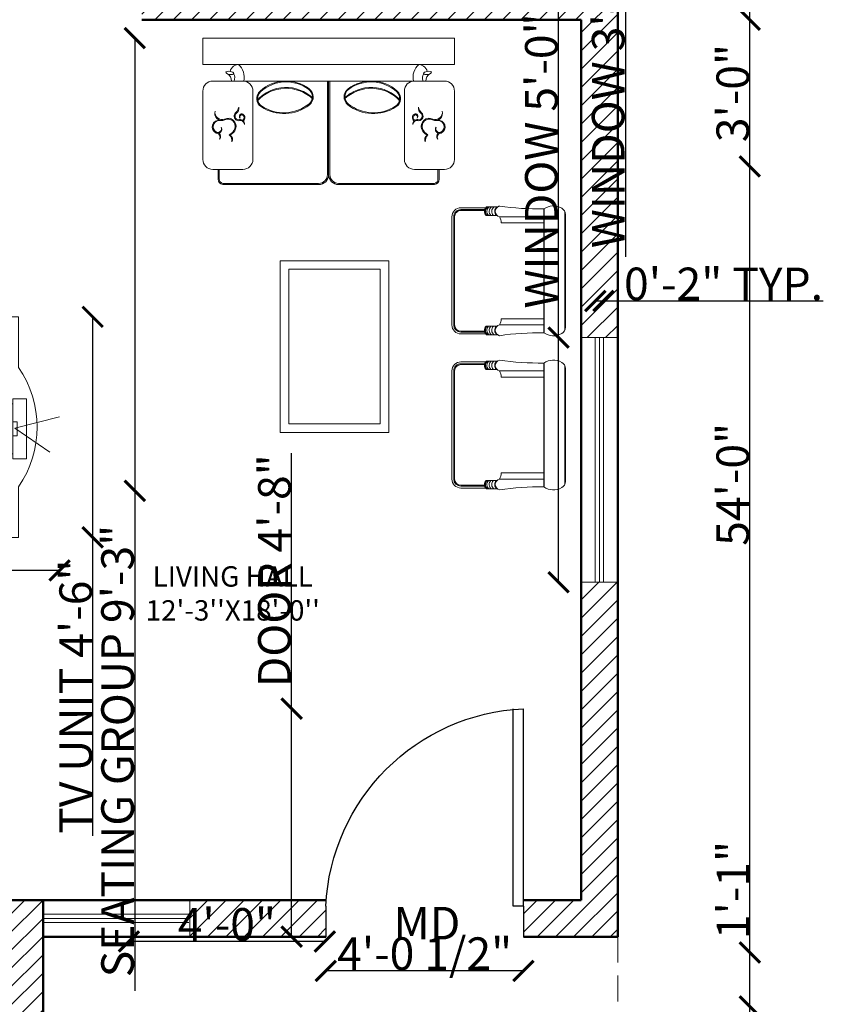
# Model space of a CAD drawing. Units: inches. Extents: x 1385 to 1778, y 1343 to 2100.
# Tile 3 of 6: x 1581 to 1778, y 1579 to 1821. Entities that reach past the tile are written whole.
import ezdxf

# ---------------------------------------------------------------- set-up
doc = ezdxf.new("R2010")
doc.units = ezdxf.units.IN
doc.linetypes.add('HIDDEN', pattern=[9.525, 6.35, -3.175])
for name, color, linetype, lineweight in [('A-ANNO-DIMS', 2, 'Continuous', 18), ('A-ANNO-TEXT', 7, 'Continuous', 25), ('A-AREA-IDEN', 7, 'Continuous', 25), ('A-FURN', 8, 'Continuous', 18), ('A-WALL-HIDN', 7, 'HIDDEN', 18), ('A-WALL-PATT', 8, 'Continuous', 13), ('Door', 150, 'Continuous', 25), ('Wall', 7, 'Continuous', 50), ('Windows', 140, 'Continuous', 18)]:
    doc.layers.add(name, color=color, linetype=linetype, lineweight=lineweight)
doc.styles.get("Standard").update_dxf_attribs({"font": 'arial.ttf'})
doc.dimstyles.get("Standard").update_dxf_attribs({"dimtxt": 8, "dimasz": 5, "dimexe": 0.18, "dimexo": 0.0625, "dimgap": 0.09, "dimtad": 1, "dimdec": 1, "dimzin": 0, "dimdsep": 46, "dimlunit": 4, "dimtxsty": 'Standard', "dimblk": 'ARCHTICK', "dimcen": 0.09, "dimse1": 1, "dimse2": 1, "dimadec": 0, "dimazin": 0, "dimtfac": 1, "dimtdec": 1, "dimtofl": 0, "dimtmove": 0, "dimatfit": 3, "dimfxl": 1, "dimtolj": 1, "dimtzin": 0, "dimarcsym": 0})

# ---------------------------------------------------------------- blocks, each defined once
blk = doc.blocks.new('AP0B05')
for p, q in [((35, 100), (35, 880)), ((75, 100), (75, 878.9)), ((35, 100), (35, -20)), ((815, 100), (815, -20))]:
    blk.add_line(p, q)
blk.add_lwpolyline([(35, 100), (75, 100)])
blk.add_arc((-2.4, 62.6), 818.3, 2.6212, 87.3788)
blk = doc.blocks.new('a12')
for p, q in [((1587.5458, -521.1815), (1587.6105, -521.1815)), ((1587.6163, -521.1869), (1587.7627, -521.1869)), ((1587.1449, -521.8934), (1587.1449, -521.226)), ((1587.1475, -521.9081), (1587.1475, -521.2114)), ((1587.2708, -521.927), (1587.2708, -521.1924)), ((1587.2727, -521.9257), (1587.2727, -521.1937)), ((1587.2727, -521.2402), (1587.535, -521.2402)), ((1587.5493, -521.232), (1587.614, -521.232)), ((1587.6223, -521.1976), (1587.7627, -521.1976)), ((1587.6236, -521.2029), (1587.7627, -521.2029)), ((1587.8, -521.8793), (1587.8, -521.2402)), ((1587.8053, -521.8793), (1587.8053, -521.2402)), ((1587.816, -521.8793), (1587.816, -521.2402)), ((1587.2727, -521.2765), (1587.5239, -521.2765)), ((1588.1896, -521.5148), (1588.1896, -522.5311)), ((1588.8309, -521.5148), (1588.1896, -521.5148)), ((1588.8309, -522.5311), (1588.8309, -521.5148)), ((1588.7801, -521.5656), (1588.2404, -521.5656)), ((1588.2404, -521.5656), (1588.2404, -522.4803)), ((1588.7801, -522.4803), (1588.7801, -521.5656)), ((1587.2727, -521.843), (1587.5239, -521.843)), ((1587.2727, -521.8793), (1587.535, -521.8793)), ((1587.5493, -521.8875), (1587.614, -521.8875)), ((1587.5458, -521.9379), (1587.6105, -521.9379)), ((1587.6163, -521.9325), (1587.7627, -521.9325)), ((1587.6223, -521.9219), (1587.7627, -521.9219)), ((1587.6236, -521.9166), (1587.7627, -521.9166)), ((1587.1475, -522.1231), (1587.1475, -522.8197)), ((1587.2708, -522.1041), (1587.2708, -522.8387)), ((1587.2727, -522.1054), (1587.2727, -522.8374)), ((1587.5458, -522.0932), (1587.6105, -522.0932)), ((1587.6163, -522.0986), (1587.7627, -522.0986)), ((1587.6223, -522.1092), (1587.7627, -522.1092)), ((1587.6236, -522.1146), (1587.7627, -522.1146)), ((1587.1449, -522.1377), (1587.1449, -522.8051)), ((1587.2727, -522.1518), (1587.535, -522.1518)), ((1587.5493, -522.1436), (1587.614, -522.1436)), ((1587.8, -522.1518), (1587.8, -522.7909)), ((1587.8053, -522.1518), (1587.8053, -522.7909)), ((1587.816, -522.1518), (1587.816, -522.7909)), ((1587.2727, -522.1881), (1587.5239, -522.1881)), ((1588.1896, -522.5311), (1588.8309, -522.5311)), ((1588.2404, -522.4803), (1588.7801, -522.4803)), ((1587.2727, -522.7546), (1587.5239, -522.7546)), ((1587.2727, -522.7909), (1587.535, -522.7909)), ((1587.5493, -522.7991), (1587.614, -522.7991)), ((1587.5458, -522.8496), (1587.6105, -522.8496)), ((1587.6163, -522.8442), (1587.7627, -522.8442)), ((1587.6223, -522.8335), (1587.7627, -522.8335)), ((1587.6236, -522.8282), (1587.7627, -522.8282)), ((1587.9193, -522.9813), (1588.4857, -522.9813)), ((1587.9193, -522.9887), (1588.4857, -522.9887)), ((1589.1705, -522.9813), (1588.6042, -522.9813)), ((1589.1705, -522.9887), (1588.6042, -522.9887)), ((1587.8908, -523.0714), (1587.8908, -523.0144)), ((1587.8982, -523.0714), (1587.8982, -523.0141)), ((1588.5375, -523.0406), (1588.5375, -523.5938)), ((1588.5449, -523.0406), (1588.5449, -523.5938)), ((1588.5449, -523.0406), (1588.5449, -523.5938)), ((1588.5523, -523.0406), (1588.5523, -523.5938)), ((1589.1916, -523.0714), (1589.1916, -523.0141)), ((1589.199, -523.0714), (1589.199, -523.0144)), ((1587.8601, -523.0714), (1588.0379, -523.0714)), ((1589.2298, -523.0714), (1589.052, -523.0714)), ((1587.8008, -523.5345), (1587.8008, -523.1307)), ((1588.0971, -523.1307), (1588.0971, -523.5345)), ((1588.9927, -523.1307), (1588.9927, -523.5345)), ((1589.2891, -523.1307), (1589.2891, -523.5345)), ((1587.8601, -523.5938), (1588.0379, -523.5938)), ((1588.0379, -523.5938), (1588.8874, -523.5938)), ((1589.2298, -523.5938), (1588.8874, -523.5938)), ((1589.2298, -523.5938), (1589.052, -523.5938)), ((1587.8008, -523.6922), (1587.8008, -523.8477)), ((1587.8008, -523.6922), (1588.0181, -523.6925)), ((1588.0181, -523.6925), (1588.8874, -523.6925)), ((1589.2895, -523.6925), (1588.8874, -523.6925)), ((1589.2895, -523.6925), (1589.2895, -523.848)), ((1587.8008, -523.8477), (1589.2895, -523.8477))]:
    blk.add_line(p, q)
for centre, radius, start, end in [((1587.1875, -521.226), 0.0426, 120.0997, 180), ((1587.2159, -521.2749), 0.0991, 54.99945, 120.0997), ((1587.2915, -519.4985), 1.6953, 269.36601, 278.25669), ((1587.5261, -521.2082), 0.0332, 285.44656, 74.55344), ((1587.5297, -521.2082), 0.0332, 314.25241, 53.67481), ((1587.5473, -521.2082), 0.0332, 314.25241, 53.67481), ((1587.5626, -521.2082), 0.0332, 314.25241, 53.67481), ((1587.5756, -521.2082), 0.0332, 314.25241, 53.67481), ((1587.585, -521.2082), 0.0332, 314.25241, 53.67481), ((1587.5885, -521.2082), 0.0332, 314.25241, 53.67481), ((1587.5909, -521.2082), 0.0332, 314.25241, 53.67481), ((1587.7627, -521.2402), 0.0533, 0, 90), ((1587.6043, -521.2812), 0.0806, 149.36468, 176.60655), ((1587.7627, -521.2402), 0.0426, 0, 90), ((1587.7627, -521.2402), 0.0373, 0, 90), ((1587.6043, -521.8382), 0.0806, 183.39345, 210.63532), ((1587.5261, -521.9112), 0.0332, 285.44656, 74.55344), ((1587.5297, -521.9112), 0.0332, 306.32519, 45.74759), ((1587.5473, -521.9112), 0.0332, 306.32519, 45.74759), ((1587.5626, -521.9112), 0.0332, 306.32519, 45.74759), ((1587.5756, -521.9112), 0.0332, 306.32519, 45.74759), ((1587.585, -521.9112), 0.0332, 306.32519, 45.74759), ((1587.5885, -521.9112), 0.0332, 306.32519, 45.74759), ((1587.5909, -521.9112), 0.0332, 306.32519, 45.74759), ((1587.7627, -521.8793), 0.0373, 270, 0), ((1587.7627, -521.8793), 0.0533, 270, 0), ((1587.7627, -521.8793), 0.0533, 270, 0), ((1587.7627, -521.8793), 0.0426, 270, 0), ((1587.1875, -521.8934), 0.0426, 180, 239.9003), ((1587.2159, -521.8445), 0.0991, 239.9003, 305.00055), ((1587.2915, -523.621), 1.6953, 81.74331, 90.63399), ((1587.1875, -522.1377), 0.0426, 120.0997, 180), ((1587.2159, -522.1866), 0.0991, 54.99945, 120.0997), ((1587.2915, -520.4102), 1.6953, 269.36601, 278.25669), ((1587.5261, -522.1199), 0.0332, 285.44656, 74.55344), ((1587.5297, -522.1199), 0.0332, 314.25241, 53.67481), ((1587.5473, -522.1199), 0.0332, 314.25241, 53.67481), ((1587.5626, -522.1199), 0.0332, 314.25241, 53.67481), ((1587.5756, -522.1199), 0.0332, 314.25241, 53.67481), ((1587.585, -522.1199), 0.0332, 314.25241, 53.67481), ((1587.5885, -522.1199), 0.0332, 314.25241, 53.67481), ((1587.5909, -522.1199), 0.0332, 314.25241, 53.67481), ((1587.7627, -522.1518), 0.0533, 0, 90), ((1587.7627, -522.1518), 0.0533, 0, 90), ((1587.7627, -522.1518), 0.0426, 0, 90), ((1587.7627, -522.1518), 0.0373, 0, 90), ((1587.6043, -522.1929), 0.0806, 149.36468, 176.60655), ((1587.6043, -522.7499), 0.0806, 183.39345, 210.63532), ((1587.1875, -522.8051), 0.0426, 180, 239.9003), ((1587.5261, -522.8229), 0.0332, 285.44656, 74.55344), ((1587.5297, -522.8229), 0.0332, 306.32519, 45.74759), ((1587.5473, -522.8229), 0.0332, 306.32519, 45.74759), ((1587.5626, -522.8229), 0.0332, 306.32519, 45.74759), ((1587.5756, -522.8229), 0.0332, 306.32519, 45.74759), ((1587.585, -522.8229), 0.0332, 306.32519, 45.74759), ((1587.5885, -522.8229), 0.0332, 306.32519, 45.74759), ((1587.5909, -522.8229), 0.0332, 306.32519, 45.74759), ((1587.7627, -522.7909), 0.0373, 270, 0), ((1587.7627, -522.7909), 0.0533, 270, 0), ((1587.7627, -522.7909), 0.0426, 270, 0), ((1587.2159, -522.7562), 0.0991, 239.9003, 305.00055), ((1587.2915, -524.5326), 1.6953, 81.74331, 90.63399), ((1587.9246, -523.0147), 0.0338, 99.00896, 179.45532), ((1587.9243, -523.0144), 0.0261, 101.02846, 180.62181), ((1588.4857, -523.0406), 0.0593, 0, 90), ((1588.4857, -523.0406), 0.0519, 0, 90), ((1588.6042, -523.0406), 0.0593, 90, 180), ((1588.6042, -523.0406), 0.0519, 90, 180), ((1589.1652, -523.0147), 0.0338, 0.54468, 80.99104), ((1589.1655, -523.0144), 0.0261, 359.37819, 78.97154), ((1587.8601, -523.1307), 0.0593, 90, 180), ((1588.0379, -523.1307), 0.0593, 0, 90), ((1589.052, -523.1307), 0.0593, 90, 180), ((1589.2298, -523.1307), 0.0593, 0, 90), ((1587.8964, -523.3224), 0.0399, 115.19964, 278.65353), ((1587.878, -523.2618), 0.0246, 273.2249, 26.32658), ((1587.8806, -523.2664), 0.0249, 311.00561, 38.72517), ((1587.8896, -523.308), 0.024, 326.9852, 72.11205), ((1587.9194, -523.2379), 0.0539, 314.74736, 4.72134), ((1587.9297, -523.3334), 0.0635, 18.04377, 64.14106), ((1587.9452, -523.2474), 0.0313, 303.93187, 26.4993), ((1587.9297, -523.3334), 0.0684, 18.04377, 61.22352), ((1589.1602, -523.3334), 0.0684, 118.77648, 161.95623), ((1589.1602, -523.3334), 0.0635, 115.85894, 161.95623), ((1589.1447, -523.2474), 0.0313, 153.5007, 236.06813), ((1589.1704, -523.2379), 0.0539, 175.27866, 225.25264), ((1589.2003, -523.308), 0.024, 107.88795, 213.0148), ((1589.2092, -523.2664), 0.0249, 141.27483, 228.99439), ((1589.2119, -523.2618), 0.0246, 153.67342, 266.7751), ((1589.1935, -523.3224), 0.0399, 261.34647, 64.80036), ((1587.8997, -523.3239), 0.0378, 118.7644, 281.17993), ((1587.8887, -523.3123), 0.0227, 337.51186, 108.42044), ((1587.95, -523.3267), 0.0471, 244.14106, 18.04377), ((1587.95, -523.3267), 0.0421, 244.14106, 18.04377), ((1588.0216, -523.3356), 0.0252, 246.46421, 356.31845), ((1588.022, -523.3415), 0.0251, 316.36053, 9.6394), ((1589.0679, -523.3415), 0.0251, 170.3606, 223.63947), ((1589.0683, -523.3356), 0.0252, 183.68155, 293.53579), ((1589.1398, -523.3267), 0.0471, 161.95623, 295.85894), ((1589.1398, -523.3267), 0.0421, 161.95623, 295.85894), ((1589.2012, -523.3123), 0.0227, 71.57956, 202.48814), ((1589.1902, -523.3239), 0.0378, 258.82007, 61.2356), ((1587.9133, -523.4026), 0.0421, 64.14106, 198.04377), ((1587.9139, -523.4076), 0.0415, 68.00293, 191.14653), ((1588.0136, -523.3861), 0.0274, 94.4509, 227.00708), ((1588.0136, -523.3861), 0.0225, 97.9146, 227.00708), ((1587.9764, -523.4327), 0.0373, 350.14408, 53.99381), ((1588.022, -523.3415), 0.0251, 242.9125, 304.68185), ((1588.0309, -523.3855), 0.014, 130.82722, 298.69388), ((1588.0317, -523.3818), 0.0122, 145.89585, 286.5587), ((1588.0265, -523.3775), 0.0182, 298.69388, 57.38696), ((1588.0265, -523.3775), 0.0232, 298.69388, 53.71752), ((1588.2799, -523.6475), 0.2459, 52.01846, 122.68708), ((1588.81, -523.6475), 0.2459, 57.31292, 127.98154), ((1589.0634, -523.3775), 0.0232, 126.28248, 241.30612), ((1589.0634, -523.3775), 0.0182, 122.61304, 241.30612), ((1589.059, -523.3855), 0.014, 241.30612, 49.17278), ((1589.0679, -523.3415), 0.0251, 235.31815, 297.0875), ((1589.0581, -523.3818), 0.0122, 253.4413, 34.10415), ((1589.1135, -523.4327), 0.0373, 126.00619, 189.85592), ((1589.0762, -523.3861), 0.0274, 312.99292, 85.5491), ((1589.0762, -523.3861), 0.0225, 312.99292, 82.0854), ((1589.1766, -523.4026), 0.0421, 341.95623, 115.85894), ((1589.1759, -523.4076), 0.0415, 348.85347, 111.99707), ((1587.9537, -523.4505), 0.0605, 10.80768, 47.00708), ((1588.1791, -523.4904), 0.0593, 122.68708, 227.67523), ((1588.1791, -523.4904), 0.0543, 122.68708, 227.67523), ((1588.2799, -523.6475), 0.241, 52.01846, 122.68708), ((1588.3947, -523.5004), 0.0543, 307.03031, 52.01846), ((1588.3947, -523.5004), 0.0593, 307.03031, 52.01846), ((1588.6951, -523.5004), 0.0593, 127.98154, 232.96969), ((1588.6951, -523.5004), 0.0543, 127.98154, 232.96969), ((1588.81, -523.6475), 0.241, 57.31292, 127.98154), ((1588.9108, -523.4904), 0.0543, 312.32477, 57.31292), ((1588.9108, -523.4904), 0.0593, 312.32477, 57.31292), ((1589.1362, -523.4505), 0.0605, 132.99292, 169.19232), ((1588.2929, -523.3227), 0.2333, 222.42727, 313.46833), ((1588.2929, -523.3227), 0.2283, 221.56925, 314.25935), ((1588.797, -523.3227), 0.2333, 226.53167, 317.57273), ((1588.797, -523.3227), 0.2283, 225.74065, 318.43075), ((1587.8601, -523.5345), 0.0593, 180, 270), ((1588.0379, -523.5345), 0.0593, 270, 0), ((1588.2929, -523.3654), 0.2283, 227.67523, 307.03031), ((1588.2929, -523.3654), 0.2234, 227.67523, 307.03031), ((1588.797, -523.3654), 0.2283, 232.96969, 312.32477), ((1588.797, -523.3654), 0.2234, 232.96969, 312.32477), ((1589.052, -523.5345), 0.0593, 180, 270), ((1589.2298, -523.5345), 0.0593, 270, 0), ((1587.9209, -523.5943), 0.0496, 301.59652, 0.58818), ((1587.9384, -523.6125), 0.0512, 330.40944, 21.39777), ((1587.9415, -523.6152), 0.1044, 312.46993, 11.85348), ((1589.1484, -523.6152), 0.1044, 168.14652, 227.53007), ((1589.1515, -523.6125), 0.0512, 158.60223, 209.59056), ((1589.169, -523.5943), 0.0496, 179.41182, 238.40348), ((1588.0181, -523.6333), 0.0593, 197.506, 270), ((1589.0717, -523.6333), 0.0593, 270, 342.494)]:
    blk.add_arc(centre, radius, start, end)
at = {"extrusion": (0, 0, -1)}
blk.add_ellipse((1587.9602, -523.6422), major_axis=(-0.023, -0.0035), ratio=0.388107, start_param=3.141593, end_param=9.424778, dxfattribs=at)
blk.add_ellipse((1589.1296, -523.6422), major_axis=(0.023, -0.0035), ratio=0.388107, start_param=3.141593, end_param=9.424778)
blk = doc.blocks.new('banghe81')
for p, q in [((-500, 3000), (0, 3000)), ((-500, 2312), (-500, 3000)), ((0, 3000), (0, 0)), ((-607, 1930), (-419, 1930)), ((-607, 1117), (-607, 1930)), ((-419, 1930), (-419, 1117)), ((-925, 1843), (-450, 1517)), ((-107, 1742), (-419, 1867)), ((-107, 1305), (-107, 1742)), ((-482, 1617), (-482, 1430)), ((-419, 1617), (-482, 1617)), ((-450, 1517), (-1057, 1361)), ((-482, 1430), (-419, 1430)), ((-419, 1180), (-107, 1305)), ((-419, 1117), (-607, 1117)), ((-500, 0), (-500, 688)), ((0, 0), (-500, 0)), ((-500, 0), (-500, 0))]:
    blk.add_line(p, q)
blk.add_arc((695, 1500), 1445, 145.7945, 214.2055)
blk = doc.blocks.new('WINDOW-GLAZING-36IN')
for p, q in [((0, 0), (0, 36)), ((1, 0), (1, 36)), ((2, 0), (2, 36))]:
    blk.add_line(p, q)
blk = doc.blocks.new('WINDOW-GLAZING-60IN')
for p, q in [((0, 0), (0, 60)), ((1, 0), (1, 60)), ((2, 0), (2, 60))]:
    blk.add_line(p, q)
blk = doc.blocks.new('_ArchTick')
at = {"color": 0, "linetype": 'ByBlock', "const_width": 0.15}
blk.add_lwpolyline([(-0.5, -0.5), (0.5, 0.5)], dxfattribs=at)
blk = doc.blocks.new('*D23')
at = {"layer": 'A-ANNO-DIMS', "color": 0, "lineweight": -2, "transparency": 16777216}
for p, q in [((1647.77, 1651.67), (1647.77, 1714.36)), ((1647.77, 1595.73), (1647.77, 1651.67))]:
    blk.add_line(p, q, dxfattribs=at)
at = {"layer": 'Defpoints', "color": 0, "transparency": 16777216}
for p in [(1647.77, 1651.67), (1656.16, 1651.67), (1656.16, 1595.73)]:
    blk.add_point(p, dxfattribs=at)
at = {"layer": 'A-ANNO-DIMS', "color": 0, "lineweight": -2, "transparency": 16777216, "xscale": 5, "yscale": 5, "zscale": 5}
for p, rotation in [((1647.77, 1651.67), 90), ((1647.77, 1595.73), 270)]:
    blk.add_blockref('_ArchTick', p, dxfattribs=dict(at, rotation=rotation))
at = {"layer": 'A-ANNO-DIMS', "color": 0, "transparency": 16777216, "insert": (1643.54, 1685.52), "char_height": 8, "attachment_point": 5, "rotation": 90}
blk.add_mtext('\\A1;DOOR 4\'-8"', dxfattribs=at)
blk = doc.blocks.new('*D24')
at = {"layer": 'A-ANNO-DIMS', "color": 0, "lineweight": -2, "transparency": 16777216}
blk.add_line((1704.65, 1587.34), (1656.16, 1587.34), dxfattribs=at)
at = {"layer": 'Defpoints', "color": 0, "transparency": 16777216}
for p in [(1656.16, 1595.73), (1704.65, 1595.73), (1656.16, 1587.34)]:
    blk.add_point(p, dxfattribs=at)
at = {"layer": 'A-ANNO-DIMS', "color": 0, "lineweight": -2, "transparency": 16777216, "xscale": 5, "yscale": 5, "zscale": 5, "rotation": 180}
blk.add_blockref('_ArchTick', (1656.16, 1587.34), dxfattribs=at)
at = {"layer": 'A-ANNO-DIMS', "color": 0, "lineweight": -2, "transparency": 16777216, "xscale": 5, "yscale": 5, "zscale": 5}
blk.add_blockref('_ArchTick', (1704.65, 1587.34), dxfattribs=at)
at = {"layer": 'A-ANNO-DIMS', "color": 0, "transparency": 16777216, "insert": (1680.41, 1591.57), "char_height": 8, "attachment_point": 5}
blk.add_mtext('\\A1;4\'-0 1/2"', dxfattribs=at)
blk = doc.blocks.new('*D27')
at = {"layer": 'A-ANNO-DIMS', "color": 0, "lineweight": -2, "transparency": 16777216}
for p, q in [((1729.67, 1904.94), (1729.67, 1868.94)), ((1729.67, 1868.94), (1729.67, 1762.53))]:
    blk.add_line(p, q, dxfattribs=at)
at = {"layer": 'Defpoints', "color": 0, "transparency": 16777216}
for p in [(1724.27, 1904.94), (1724.27, 1868.94), (1729.67, 1868.94)]:
    blk.add_point(p, dxfattribs=at)
at = {"layer": 'A-ANNO-DIMS', "color": 0, "lineweight": -2, "transparency": 16777216, "xscale": 5, "yscale": 5, "zscale": 5}
for p, rotation in [((1729.67, 1904.94), 90), ((1729.67, 1868.94), 270)]:
    blk.add_blockref('_ArchTick', p, dxfattribs=dict(at, rotation=rotation))
at = {"layer": 'A-ANNO-DIMS', "color": 0, "transparency": 16777216, "insert": (1725.44, 1813.24), "char_height": 8, "attachment_point": 5, "rotation": 90}
blk.add_mtext('\\A1;WINDOW 3\'-0" TYP.', dxfattribs=at)
blk = doc.blocks.new('*D31')
at = {"layer": 'A-ANNO-DIMS', "color": 0, "lineweight": -2, "transparency": 16777216}
for p, q in [((1713.27, 1742.73), (1713.27, 1849.15)), ((1713.27, 1682.73), (1713.27, 1742.73))]:
    blk.add_line(p, q, dxfattribs=at)
at = {"layer": 'Defpoints', "color": 0, "transparency": 16777216}
for p in [(1713.27, 1742.73), (1722.27, 1742.73), (1722.27, 1682.73)]:
    blk.add_point(p, dxfattribs=at)
at = {"layer": 'A-ANNO-DIMS', "color": 0, "lineweight": -2, "transparency": 16777216, "xscale": 5, "yscale": 5, "zscale": 5}
for p, rotation in [((1713.27, 1742.73), 90), ((1713.27, 1682.73), 270)]:
    blk.add_blockref('_ArchTick', p, dxfattribs=dict(at, rotation=rotation))
at = {"layer": 'A-ANNO-DIMS', "color": 0, "transparency": 16777216, "insert": (1709.04, 1798.44), "char_height": 8, "attachment_point": 5, "rotation": 90}
blk.add_mtext('\\A1;WINDOW 5\'-0" TYP.', dxfattribs=at)
blk = doc.blocks.new('*D32')
at = {"layer": 'A-ANNO-DIMS', "color": 0, "lineweight": -2, "transparency": 16777216}
for p, q in [((1722.27, 1751.73), (1724.27, 1751.73)), ((1724.27, 1751.73), (1778.22, 1751.73))]:
    blk.add_line(p, q, dxfattribs=at)
at = {"layer": 'Defpoints', "color": 0, "transparency": 16777216}
for p in [(1724.27, 1751.73), (1722.27, 1742.73), (1724.27, 1742.73)]:
    blk.add_point(p, dxfattribs=at)
at = {"layer": 'A-ANNO-DIMS', "color": 0, "lineweight": -2, "transparency": 16777216, "xscale": 5, "yscale": 5, "zscale": 5, "rotation": 180}
blk.add_blockref('_ArchTick', (1722.27, 1751.73), dxfattribs=at)
at = {"layer": 'A-ANNO-DIMS', "color": 0, "lineweight": -2, "transparency": 16777216, "xscale": 5, "yscale": 5, "zscale": 5}
blk.add_blockref('_ArchTick', (1724.27, 1751.73), dxfattribs=at)
at = {"layer": 'A-ANNO-DIMS', "color": 0, "transparency": 16777216, "insert": (1753.74, 1755.91), "char_height": 8, "attachment_point": 5}
blk.add_mtext('\\A1;0\'-2" TYP.', dxfattribs=at)
blk = doc.blocks.new('*D40')
at = {"layer": 'A-ANNO-DIMS', "color": 0, "lineweight": -2, "transparency": 16777216}
blk.add_line((1655.9, 1594.57), (1607.85, 1594.57), dxfattribs=at)
at = {"layer": 'Defpoints', "color": 0, "transparency": 16777216}
for p in [(1607.85, 1594.57), (1607.85, 1574.58), (1655.9, 1574.58)]:
    blk.add_point(p, dxfattribs=at)
at = {"layer": 'A-ANNO-DIMS', "color": 0, "lineweight": -2, "transparency": 16777216, "xscale": 5, "yscale": 5, "zscale": 5, "rotation": 180}
blk.add_blockref('_ArchTick', (1607.85, 1594.57), dxfattribs=at)
at = {"layer": 'A-ANNO-DIMS', "color": 0, "lineweight": -2, "transparency": 16777216, "xscale": 5, "yscale": 5, "zscale": 5}
blk.add_blockref('_ArchTick', (1655.9, 1594.57), dxfattribs=at)
at = {"layer": 'A-ANNO-DIMS', "color": 0, "transparency": 16777216, "insert": (1631.88, 1598.75), "char_height": 8, "attachment_point": 5}
blk.add_mtext('\\A1;4\'-0"', dxfattribs=at)
blk = doc.blocks.new('*D41')
at = {"layer": 'A-ANNO-DIMS', "color": 0, "lineweight": -2, "transparency": 16777216}
for p, q in [((1609.29, 1816.23), (1609.29, 1705.12)), ((1609.29, 1705.12), (1609.29, 1582.46))]:
    blk.add_line(p, q, dxfattribs=at)
at = {"layer": 'Defpoints', "color": 0, "transparency": 16777216}
for p in [(1625.96, 1816.23), (1609.29, 1705.12), (1625.96, 1705.12)]:
    blk.add_point(p, dxfattribs=at)
at = {"layer": 'A-ANNO-DIMS', "color": 0, "lineweight": -2, "transparency": 16777216, "xscale": 5, "yscale": 5, "zscale": 5}
for p, rotation in [((1609.29, 1816.23), 90), ((1609.29, 1705.12), 270)]:
    blk.add_blockref('_ArchTick', p, dxfattribs=dict(at, rotation=rotation))
at = {"layer": 'A-ANNO-DIMS', "color": 0, "transparency": 16777216, "insert": (1605.06, 1641.29), "char_height": 8, "attachment_point": 5, "rotation": 90}
blk.add_mtext('\\A1;SEATING GROUP 9\'-3"', dxfattribs=at)
blk = doc.blocks.new('*D42')
at = {"layer": 'A-ANNO-DIMS', "color": 0, "lineweight": -2, "transparency": 16777216}
blk.add_line((1714.93, 1832.89), (1625.96, 1832.89), dxfattribs=at)
at = {"layer": 'Defpoints', "color": 0, "transparency": 16777216}
for p in [(1625.96, 1832.89), (1625.96, 1816.23), (1714.93, 1816.23)]:
    blk.add_point(p, dxfattribs=at)
at = {"layer": 'A-ANNO-DIMS', "color": 0, "lineweight": -2, "transparency": 16777216, "xscale": 5, "yscale": 5, "zscale": 5, "rotation": 180}
blk.add_blockref('_ArchTick', (1625.96, 1832.89), dxfattribs=at)
at = {"layer": 'A-ANNO-DIMS', "color": 0, "lineweight": -2, "transparency": 16777216, "xscale": 5, "yscale": 5, "zscale": 5}
blk.add_blockref('_ArchTick', (1714.93, 1832.89), dxfattribs=at)
at = {"layer": 'A-ANNO-DIMS', "color": 0, "transparency": 16777216, "insert": (1670.44, 1837.05), "char_height": 8, "attachment_point": 5}
blk.add_mtext('\\A1;7\'-5"', dxfattribs=at)
blk = doc.blocks.new('*D47')
at = {"layer": 'A-ANNO-DIMS', "color": 0, "lineweight": -2, "transparency": 16777216}
for p, q in [((1598.95, 1747.83), (1598.95, 1693.73)), ((1598.95, 1693.73), (1598.95, 1620.51))]:
    blk.add_line(p, q, dxfattribs=at)
at = {"layer": 'Defpoints', "color": 0, "transparency": 16777216}
for p in [(1590.84, 1747.83), (1590.84, 1693.73), (1598.95, 1693.73)]:
    blk.add_point(p, dxfattribs=at)
at = {"layer": 'A-ANNO-DIMS', "color": 0, "lineweight": -2, "transparency": 16777216, "xscale": 5, "yscale": 5, "zscale": 5}
for p, rotation in [((1598.95, 1747.83), 90), ((1598.95, 1693.73), 270)]:
    blk.add_blockref('_ArchTick', p, dxfattribs=dict(at, rotation=rotation))
at = {"layer": 'A-ANNO-DIMS', "color": 0, "transparency": 16777216, "insert": (1594.78, 1654.62), "char_height": 8, "attachment_point": 5, "rotation": 90}
blk.add_mtext('\\A1;TV UNIT 4\'-6"', dxfattribs=at)
blk = doc.blocks.new('*D48')
at = {"layer": 'A-ANNO-DIMS', "color": 0, "lineweight": -2, "transparency": 16777216}
for p, q in [((1571.77, 1685.61), (1546.08, 1685.61)), ((1590.84, 1685.61), (1571.77, 1685.61))]:
    blk.add_line(p, q, dxfattribs=at)
at = {"layer": 'Defpoints', "color": 0, "transparency": 16777216}
for p in [(1571.77, 1693.73), (1590.84, 1693.73), (1571.77, 1685.61)]:
    blk.add_point(p, dxfattribs=at)
at = {"layer": 'A-ANNO-DIMS', "color": 0, "lineweight": -2, "transparency": 16777216, "xscale": 5, "yscale": 5, "zscale": 5, "rotation": 180}
blk.add_blockref('_ArchTick', (1571.77, 1685.61), dxfattribs=at)
at = {"layer": 'A-ANNO-DIMS', "color": 0, "lineweight": -2, "transparency": 16777216, "xscale": 5, "yscale": 5, "zscale": 5}
blk.add_blockref('_ArchTick', (1590.84, 1685.61), dxfattribs=at)
at = {"layer": 'A-ANNO-DIMS', "color": 0, "transparency": 16777216, "insert": (1556.43, 1689.72), "char_height": 8, "attachment_point": 5}
blk.add_mtext('\\A1;1\'-7"', dxfattribs=at)
blk = doc.blocks.new('*D50')
at = {"layer": 'A-ANNO-DIMS', "color": 0, "lineweight": -2, "transparency": 16777216}
blk.add_line((1760.18, 1382.73), (1760.18, 2030.73), dxfattribs=at)
at = {"layer": 'Defpoints', "color": 0, "transparency": 16777216}
for p in [(1727.77, 2030.73), (1760.18, 2030.73), (1727.77, 1382.73)]:
    blk.add_point(p, dxfattribs=at)
at = {"layer": 'A-ANNO-DIMS', "color": 0, "lineweight": -2, "transparency": 16777216, "xscale": 5, "yscale": 5, "zscale": 5}
for p, rotation in [((1760.18, 2030.73), 90), ((1760.18, 1382.73), 270)]:
    blk.add_blockref('_ArchTick', p, dxfattribs=dict(at, rotation=rotation))
at = {"layer": 'A-ANNO-DIMS', "color": 0, "transparency": 16777216, "insert": (1756, 1706.73), "char_height": 8, "attachment_point": 5, "rotation": 90}
blk.add_mtext('\\A1;54\'-0"', dxfattribs=at)
blk = doc.blocks.new('*D55')
at = {"layer": 'A-ANNO-DIMS', "color": 0, "lineweight": -2, "transparency": 16777216}
blk.add_line((1401.37, 1604.73), (1401.37, 1682.73), dxfattribs=at)
at = {"layer": 'Defpoints', "color": 0, "transparency": 16777216}
for p in [(1401.37, 1682.73), (1718.77, 1682.73), (1718.77, 1604.73)]:
    blk.add_point(p, dxfattribs=at)
at = {"layer": 'A-ANNO-DIMS', "color": 0, "lineweight": -2, "transparency": 16777216, "xscale": 5, "yscale": 5, "zscale": 5}
for p, rotation in [((1401.37, 1682.73), 90), ((1401.37, 1604.73), 270)]:
    blk.add_blockref('_ArchTick', p, dxfattribs=dict(at, rotation=rotation))
at = {"layer": 'A-ANNO-DIMS', "color": 0, "transparency": 16777216, "insert": (1397.19, 1643.73), "char_height": 8, "attachment_point": 5, "rotation": 90}
blk.add_mtext('\\A1;6\'-6"', dxfattribs=at)
blk = doc.blocks.new('*D61')
at = {"layer": 'A-ANNO-DIMS', "color": 0, "lineweight": -2, "transparency": 16777216}
blk.add_line((1586.77, 2063.14), (1708.55, 2063.14), dxfattribs=at)
at = {"layer": 'Defpoints', "color": 0, "transparency": 16777216}
for p in [(1708.55, 2063.14), (1586.77, 1382.73), (1708.55, 1382.73)]:
    blk.add_point(p, dxfattribs=at)
at = {"layer": 'A-ANNO-DIMS', "color": 0, "lineweight": -2, "transparency": 16777216, "xscale": 5, "yscale": 5, "zscale": 5, "rotation": 180}
blk.add_blockref('_ArchTick', (1586.77, 2063.14), dxfattribs=at)
at = {"layer": 'A-ANNO-DIMS', "color": 0, "lineweight": -2, "transparency": 16777216, "xscale": 5, "yscale": 5, "zscale": 5}
blk.add_blockref('_ArchTick', (1708.55, 2063.14), dxfattribs=at)
at = {"layer": 'A-ANNO-DIMS', "color": 0, "transparency": 16777216, "insert": (1647.66, 2067.31), "char_height": 8, "attachment_point": 5}
blk.add_mtext('\\A1;10\'-2"', dxfattribs=at)
blk = doc.blocks.new('*D67')
at = {"layer": 'A-ANNO-DIMS', "color": 0, "lineweight": -2, "transparency": 16777216}
for p, q in [((1513.34, 2063.14), (1546.08, 2063.14)), ((1546.08, 2063.14), (1591.31, 2063.14))]:
    blk.add_line(p, q, dxfattribs=at)
at = {"layer": 'Defpoints', "color": 0, "transparency": 16777216}
for p in [(1546.08, 2063.14), (1513.34, 1595.73), (1546.08, 1595.73)]:
    blk.add_point(p, dxfattribs=at)
at = {"layer": 'A-ANNO-DIMS', "color": 0, "lineweight": -2, "transparency": 16777216, "xscale": 5, "yscale": 5, "zscale": 5, "rotation": 180}
blk.add_blockref('_ArchTick', (1513.34, 2063.14), dxfattribs=at)
at = {"layer": 'A-ANNO-DIMS', "color": 0, "lineweight": -2, "transparency": 16777216, "xscale": 5, "yscale": 5, "zscale": 5}
blk.add_blockref('_ArchTick', (1546.08, 2063.14), dxfattribs=at)
at = {"layer": 'A-ANNO-DIMS', "color": 0, "transparency": 16777216, "insert": (1571.19, 2067.37), "char_height": 8, "attachment_point": 5}
blk.add_mtext('\\A1;2\'-8 1/2"', dxfattribs=at)
blk = doc.blocks.new('*D68')
at = {"layer": 'A-ANNO-DIMS', "color": 0, "lineweight": -2, "transparency": 16777216}
for p, q in [((1704.65, 1350.33), (1727.77, 1350.33)), ((1727.77, 1350.33), (1759.68, 1350.33))]:
    blk.add_line(p, q, dxfattribs=at)
at = {"layer": 'Defpoints', "color": 0, "transparency": 16777216}
for p in [(1704.65, 1595.73), (1727.77, 1595.73), (1727.77, 1350.33)]:
    blk.add_point(p, dxfattribs=at)
at = {"layer": 'A-ANNO-DIMS', "color": 0, "lineweight": -2, "transparency": 16777216, "xscale": 5, "yscale": 5, "zscale": 5, "rotation": 180}
blk.add_blockref('_ArchTick', (1704.65, 1350.33), dxfattribs=at)
at = {"layer": 'A-ANNO-DIMS', "color": 0, "lineweight": -2, "transparency": 16777216, "xscale": 5, "yscale": 5, "zscale": 5}
blk.add_blockref('_ArchTick', (1727.77, 1350.33), dxfattribs=at)
at = {"layer": 'A-ANNO-DIMS', "color": 0, "transparency": 16777216, "insert": (1746.23, 1354.44), "char_height": 8, "attachment_point": 5}
blk.add_mtext('\\A1;1\'-11"', dxfattribs=at)
blk = doc.blocks.new('*D76')
at = {"layer": 'A-ANNO-DIMS', "color": 0, "lineweight": -2, "transparency": 16777216}
for p, q in [((1711.39, 1350.33), (1718.77, 1350.33)), ((1718.77, 1350.33), (1763.86, 1350.33))]:
    blk.add_line(p, q, dxfattribs=at)
at = {"layer": 'Defpoints', "color": 0, "transparency": 16777216}
for p in [(1711.39, 1970.73), (1718.77, 1970.73), (1718.77, 1350.33)]:
    blk.add_point(p, dxfattribs=at)
at = {"layer": 'A-ANNO-DIMS', "color": 0, "lineweight": -2, "transparency": 16777216, "xscale": 5, "yscale": 5, "zscale": 5, "rotation": 180}
blk.add_blockref('_ArchTick', (1711.39, 1350.33), dxfattribs=at)
at = {"layer": 'A-ANNO-DIMS', "color": 0, "lineweight": -2, "transparency": 16777216, "xscale": 5, "yscale": 5, "zscale": 5}
blk.add_blockref('_ArchTick', (1718.77, 1350.33), dxfattribs=at)
at = {"layer": 'A-ANNO-DIMS', "color": 0, "transparency": 16777216, "insert": (1743.82, 1354.56), "char_height": 8, "attachment_point": 5}
blk.add_mtext('\\A1;0\'-7 1/2"', dxfattribs=at)
blk = doc.blocks.new('*D79')
at = {"layer": 'A-ANNO-DIMS', "color": 0, "lineweight": -2, "transparency": 16777216}
blk.add_line((1760.18, 1784.73), (1760.18, 1820.73), dxfattribs=at)
at = {"layer": 'Defpoints', "color": 0, "transparency": 16777216}
for p in [(1508.77, 1820.73), (1760.18, 1820.73), (1508.77, 1784.73)]:
    blk.add_point(p, dxfattribs=at)
at = {"layer": 'A-ANNO-DIMS', "color": 0, "lineweight": -2, "transparency": 16777216, "xscale": 5, "yscale": 5, "zscale": 5}
for p, rotation in [((1760.18, 1820.73), 90), ((1760.18, 1784.73), 270)]:
    blk.add_blockref('_ArchTick', p, dxfattribs=dict(at, rotation=rotation))
at = {"layer": 'A-ANNO-DIMS', "color": 0, "transparency": 16777216, "insert": (1756, 1802.73), "char_height": 8, "attachment_point": 5, "rotation": 90}
blk.add_mtext('\\A1;3\'-0"', dxfattribs=at)
blk = doc.blocks.new('*D81')
at = {"layer": 'A-ANNO-DIMS', "color": 0, "lineweight": -2, "transparency": 16777216}
for p, q in [((1760.18, 1591.85), (1760.18, 1617.54)), ((1760.18, 1578.65), (1760.18, 1591.85))]:
    blk.add_line(p, q, dxfattribs=at)
at = {"layer": 'Defpoints', "color": 0, "transparency": 16777216}
for p in [(1510.83, 1591.85), (1760.18, 1591.85), (1510.83, 1578.65)]:
    blk.add_point(p, dxfattribs=at)
at = {"layer": 'A-ANNO-DIMS', "color": 0, "lineweight": -2, "transparency": 16777216, "xscale": 5, "yscale": 5, "zscale": 5}
for p, rotation in [((1760.18, 1591.85), 90), ((1760.18, 1578.65), 270)]:
    blk.add_blockref('_ArchTick', p, dxfattribs=dict(at, rotation=rotation))
at = {"layer": 'A-ANNO-DIMS', "color": 0, "transparency": 16777216, "insert": (1756.07, 1607.19), "char_height": 8, "attachment_point": 5, "rotation": 90}
blk.add_mtext('\\A1;1\'-1"', dxfattribs=at)

msp = doc.modelspace()

# ---------------------------------------------------------------- hatches: boundary and pattern name
at = {"layer": 'A-WALL-PATT', "transparency": 33554585}
h = msp.add_hatch(dxfattribs=at)
h.set_pattern_fill('ANSI31', color=256)
h.paths.add_polyline_path([(1522.75, 2030.73), (1433.77, 2030.73), (1433.77, 1900.6), (1442.77, 1900.6), (1442.77, 2021.73), (1522.75, 2021.73)])
h.paths.add_polyline_path([(1591.32, 2030.73), (1558.75, 2030.73), (1558.75, 2021.73), (1571.77, 2021.73), (1591.32, 2021.73)], flags=17)
h.paths.add_polyline_path([(1664.16, 2030.73), (1615.32, 2030.73), (1615.32, 2021.73), (1646.77, 2021.73), (1646.77, 1970.73), (1571.77, 1970.73), (1571.77, 1990.51, -0.048507), (1566.67, 1989.78), (1562.77, 1989.78), (1562.77, 1829.73), (1557.76, 1829.73), (1557.76, 1826.48), (1557.76, 1820.73), (1578.09, 1820.73), (1578.09, 1825.8), (1578.09, 1829.73), (1571.77, 1829.73), (1571.77, 1961.73), (1686.02, 1961.73), (1686.02, 1965.64, -0.048507), (1686.76, 1970.73), (1650.77, 1970.73), (1650.77, 2021.73), (1664.16, 2021.73)])
h.paths.add_polyline_path([(1727.77, 2030.73), (1688.16, 2030.73), (1688.16, 2021.73), (1718.77, 2021.73), (1718.77, 1970.73), (1711.39, 1970.73), (1711.39, 1965.64), (1711.39, 1961.73), (1718.77, 1961.73), (1718.77, 1904.94), (1727.77, 1904.94)])
h.paths.add_polyline_path([(1727.77, 1868.94), (1718.77, 1868.94), (1718.77, 1829.73), (1610.61, 1829.73, -0.028655), (1611.02, 1825.8), (1611.02, 1820.73), (1718.77, 1820.73), (1718.77, 1742.73), (1727.77, 1742.73)])
h.paths.add_polyline_path([(1520.45, 1826.48, -0.020905), (1520.74, 1829.73), (1442.77, 1829.73), (1442.77, 1840.6), (1433.77, 1840.6), (1433.77, 1794.33), (1442.77, 1794.33), (1442.77, 1820.73), (1502.77, 1820.73), (1502.77, 1760.73), (1497.07, 1760.73), (1497.07, 1759.8), (1497.07, 1754.73), (1508.77, 1754.73), (1508.77, 1778.73), (1562.77, 1778.73), (1562.77, 1656.82), (1571.77, 1656.82), (1571.77, 1784.73), (1508.77, 1784.73), (1508.77, 1820.73), (1520.45, 1820.73)])
h.paths.add_polyline_path([(1442.77, 1770.33), (1433.77, 1770.33), (1433.77, 1683.46), (1442.77, 1683.46)], flags=17)
h.paths.add_polyline_path([(1656.16, 1603.19, -0.007591), (1656.26, 1604.73), (1622.77, 1604.73), (1622.77, 1595.73), (1656.16, 1595.73)])
h.paths.add_polyline_path([(1727.77, 1682.73), (1718.77, 1682.73), (1718.77, 1604.73), (1704.65, 1604.73), (1704.65, 1603.19), (1704.65, 1595.73), (1727.77, 1595.73)])
h.paths.add_polyline_path([(1513.34, 1595.73), (1513.34, 1604.73), (1442.77, 1604.73), (1442.77, 1647.46), (1433.77, 1647.46), (1433.77, 1531.33), (1442.77, 1531.33), (1442.77, 1595.73)])
h.paths.add_polyline_path([(1546.08, 1604.73), (1546.08, 1595.73), (1577.77, 1595.73), (1577.77, 1472.73), (1541.77, 1472.73), (1541.77, 1523.73), (1537.77, 1523.73), (1537.77, 1472.73), (1442.77, 1472.73), (1442.77, 1495.33), (1433.77, 1495.33), (1433.77, 1382.73), (1586.77, 1382.73), (1586.77, 1391.73), (1442.77, 1391.73), (1442.77, 1463.73), (1586.77, 1463.73), (1586.77, 1604.73)])

# ---------------------------------------------------------------- linework, layer by layer
at = {"layer": 'A-WALL-HIDN'}
msp.add_line((1727.77, 1595.73), (1727.77, 1382.73), dxfattribs=at)
at = {"layer": 'Wall'}
for p, q in [((1727.77, 2030.73), (1727.77, 1595.73)), ((1611.02, 1820.73), (1718.77, 1820.73)), ((1718.77, 1820.73), (1718.77, 1604.73)), ((1546.08, 1604.73), (1656.26, 1604.73)), ((1586.77, 1604.73), (1586.77, 1463.73)), ((1704.65, 1604.73), (1718.77, 1604.73)), ((1586.77, 1595.73), (1656.16, 1595.73)), ((1704.65, 1595.73), (1727.77, 1595.73))]:
    msp.add_line(p, q, dxfattribs=at)
at = {"layer": 'Windows'}
for points in [[(1718.77, 1682.73), (1718.77, 1742.73), (1727.77, 1742.73), (1727.77, 1682.73)], [(1586.77, 1604.73), (1622.77, 1604.73), (1622.77, 1595.73), (1586.77, 1595.73)]]:
    msp.add_lwpolyline(points, close=True, dxfattribs=at)

# ---------------------------------------------------------------- block references
at = {"layer": 'A-FURN', "rotation": 180}
for name, p, xscale, yscale, zscale in [('a12', (67559.45, -19916.21), 41.48614187593929, 41.48614187593929, 41.48614187593929), ('banghe81', (1571.77, 1747.83), 0.0180362713339597, 0.0180362713339597, 0.0180362713339597)]:
    msp.add_blockref(name, p, dxfattribs=dict(at, xscale=xscale, yscale=yscale, zscale=zscale))
at = {"layer": 'Door', "xscale": -0.0621555836634118, "yscale": 0.0621555836634118, "zscale": 0.0621555836634118}
msp.add_blockref('AP0B05', (1706.82, 1596.98), dxfattribs=at)
at = {"layer": 'Windows'}
msp.add_blockref('WINDOW-GLAZING-60IN', (1722.27, 1682.73), dxfattribs=at)
at = {"layer": 'Windows', "rotation": 90.0000000000022}
msp.add_blockref('WINDOW-GLAZING-36IN', (1622.57, 1599.23), dxfattribs=at)

# ---------------------------------------------------------------- texts
at = {"layer": 'A-ANNO-TEXT'}
msp.add_text('MD', height=8, dxfattribs=at).set_placement((1672.79, 1595.06))
at = {"layer": 'A-AREA-IDEN', "insert": (1608.18, 1686.63), "char_height": 5, "attachment_point": 1}
msp.add_mtext_dynamic_manual_height_columns("\\pxqc;LIVING HALL\\P12'-3''X18'-0''", width=50.3036, gutter_width=12.5, heights=[0], dxfattribs=at)

# ---------------------------------------------------------------- dimensions: what is measured, and where the dimension line sits
at = {"layer": 'A-ANNO-DIMS'}
for base, p1, p2, picture, middle in [((1546.08, 2063.14), (1513.34, 1595.73), (1546.08, 1595.73), '*D67', (1571.19, 2067.37)), ((1708.55, 2063.14), (1586.77, 1382.73), (1708.55, 1382.73), '*D61', (1647.66, 2067.31)), ((1718.77, 1350.33), (1711.39, 1970.73), (1718.77, 1970.73), '*D76', (1743.82, 1354.56)), ((1727.77, 1350.33), (1704.65, 1595.73), (1727.77, 1595.73), '*D68', (1746.23, 1354.44))]:
    dim = msp.add_linear_dim(base=base, p1=p1, p2=p2, dimstyle='Standard', override={"dimdec": 1, "dimlfac": 1, "dimrnd": 0, "dimzin": 1, "dimdsep": 46, "dimlunit": 4, "dimfrac": 2}, dxfattribs=at)
    dim.commit()
    dim.dimension.update_dxf_attribs({"geometry": picture, "text_midpoint": middle})
for base, p1, p2, angle, picture, middle in [((1760.18, 2030.73), (1727.77, 1382.73), (1727.77, 2030.73), 90, '*D50', (1756, 1706.73)), ((1625.96, 1832.89), (1714.93, 1816.23), (1625.96, 1816.23), 180, '*D42', (1670.44, 1837.05)), ((1760.18, 1820.73), (1508.77, 1784.73), (1508.77, 1820.73), 90, '*D79', (1756, 1802.73)), ((1571.77, 1685.61), (1590.84, 1693.73), (1571.77, 1693.73), 180, '*D48', (1556.43, 1689.72)), ((1401.37, 1682.73), (1718.77, 1604.73), (1718.77, 1682.73), 90, '*D55', (1397.19, 1643.73)), ((1760.18, 1591.85), (1510.83, 1578.65), (1510.83, 1591.85), 90, '*D81', (1756.07, 1607.19)), ((1607.8471, 1594.5714), (1655.904, 1574.5804), (1607.8471, 1574.5804), 180, '*D40', (1631.8756, 1598.746)), ((1656.16, 1587.34), (1704.65, 1595.73), (1656.16, 1595.73), 180, '*D24', (1680.41, 1591.57))]:
    dim = msp.add_linear_dim(base=base, p1=p1, p2=p2, angle=angle, dimstyle='Standard', override={"dimdec": 1, "dimlfac": 1, "dimrnd": 0, "dimzin": 1, "dimdsep": 46, "dimlunit": 4, "dimfrac": 2}, dxfattribs=at)
    dim.commit()
    dim.dimension.update_dxf_attribs({"geometry": picture, "text_midpoint": middle})
for base, p1, p2, angle, text, picture, middle in [((1729.67, 1868.94), (1724.27, 1904.94), (1724.27, 1868.94), 270, 'WINDOW <> TYP.', '*D27', (1725.44, 1813.24)), ((1713.27, 1742.73), (1722.27, 1682.73), (1722.27, 1742.73), 90, 'WINDOW <> TYP.', '*D31', (1709.04, 1798.44)), ((1609.29, 1705.12), (1625.96, 1816.23), (1625.96, 1705.12), 270, 'SEATING GROUP <>', '*D41', (1605.06, 1641.29)), ((1598.95, 1693.73), (1590.84, 1747.83), (1590.84, 1693.73), 270, 'TV UNIT <>', '*D47', (1594.78, 1654.62)), ((1647.77, 1651.67), (1656.16, 1595.73), (1656.16, 1651.67), 90, 'DOOR <>', '*D23', (1643.54, 1685.52))]:
    dim = msp.add_linear_dim(base=base, p1=p1, p2=p2, angle=angle, text=text, dimstyle='Standard', override={"dimdec": 1, "dimlfac": 1, "dimrnd": 0, "dimzin": 1, "dimdsep": 46, "dimlunit": 4, "dimfrac": 2}, dxfattribs=at)
    dim.commit()
    dim.dimension.update_dxf_attribs({"geometry": picture, "text_midpoint": middle})
dim = msp.add_linear_dim(base=(1724.27, 1751.73), p1=(1722.27, 1742.73), p2=(1724.27, 1742.73), text='<> TYP.', dimstyle='Standard', override={"dimdec": 1, "dimlfac": 1, "dimrnd": 0, "dimzin": 1, "dimdsep": 46, "dimlunit": 4, "dimfrac": 2}, dxfattribs=at)
dim.commit()
dim.dimension.update_dxf_attribs({"geometry": '*D32', "text_midpoint": (1753.74, 1755.91)})

doc.saveas('drawing.dxf')
